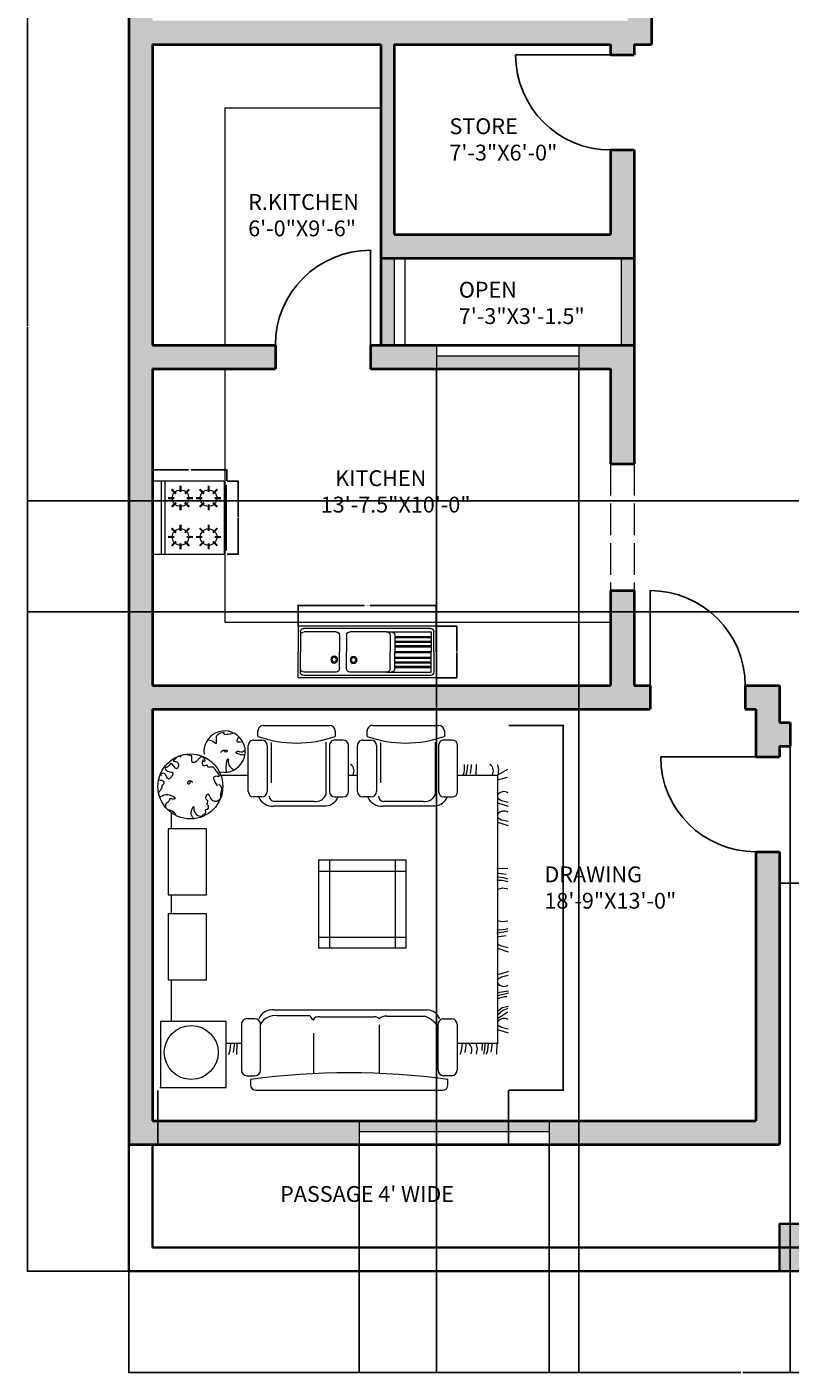
# Model space of a CAD drawing. Units: inches. Extents: x 2985 to 3527, y 3685 to 4528.
# Tile 1 of 5: x 2985 to 3274, y 3685 to 4195. Entities that reach past the tile are written whole.
import ezdxf

# ---------------------------------------------------------------- set-up
doc = ezdxf.new("R2010")
doc.units = ezdxf.units.IN
doc.linetypes.add('ACAD_ISO02W100', pattern=[15, 12, -3])
for name, color, linetype, lineweight in [('A-ANNO-DIMS', 2, 'Continuous', 18), ('A-AREA-IDEN', 7, 'Continuous', 25), ('A-EQPM', 8, 'Continuous', 18), ('A-FLOR-CASE', 9, 'Continuous', 20), ('A-FLOR-EDGE', 7, 'Continuous', 25), ('A-FLOR-FIXT', 9, 'Continuous', 18), ('A-FURN', 8, 'Continuous', 18), ('A-GLAZ', 4, 'Continuous', 18), ('A-SITE-WALL', 7, 'Continuous', 35), ('A-WALL', 7, 'Continuous', 40), ('A-WALL-OVHD', 7, 'ACAD_ISO02W100', 18), ('A-WALL-PATT', 8, 'Continuous', 13), ('door', 4, 'Continuous', 25)]:
    doc.layers.add(name, color=color, linetype=linetype, lineweight=lineweight)
doc.layers.add('A-GLAZ-PATT', color=241, linetype='Continuous', lineweight=13, true_color=0xf7abae)
doc.styles.get("Standard").update_dxf_attribs({"font": 'arial.ttf'})
doc.dimstyles.get("Standard").update_dxf_attribs({"dimtxt": 0.18, "dimasz": 0.18, "dimexe": 0.18, "dimexo": 0.0625, "dimgap": 0.09, "dimtad": 0, "dimtih": 1, "dimtoh": 1, "dimdec": 4, "dimzin": 0, "dimdsep": 46, "dimtxsty": 'Standard', "dimcen": 0.09, "dimadec": 0, "dimazin": 0, "dimtfac": 1, "dimtdec": 4, "dimtofl": 0, "dimtmove": 0, "dimatfit": 3, "dimfxl": 1, "dimtolj": 1, "dimtzin": 0, "dimarcsym": 0})

# ---------------------------------------------------------------- blocks, each defined once
blk = doc.blocks.new('A$C5E580471')
at = {"ltscale": 1000}
for p, q in [((0, 450), (0, 225)), ((1200, 450), (0, 450)), ((20, 400), (20, 225)), ((22, 370), (22, 225)), ((1150, 430), (50, 430)), ((331, 400), (52, 400)), ((361, 370), (361, 225)), ((421, 370), (421, 225)), ((770, 400), (451, 400)), ((770, 400), (1156, 400)), ((800, 370), (800, 225)), ((840, 370), (840, 225)), ((840, 360), (1156, 360)), ((1156, 400), (1156, 225)), ((1180, 225), (1180, 400)), ((1200, 225), (1200, 450)), ((840, 350), (1156, 350)), ((840, 320), (1156, 320)), ((840, 310), (1156, 310)), ((840, 280), (1156, 280)), ((840, 270), (1156, 270)), ((0, 0), (0, 225)), ((20, 50), (20, 225)), ((22, 80), (22, 225)), ((361, 80), (361, 225)), ((361, 80), (361, 225)), ((421, 80), (421, 225)), ((800, 80), (800, 225)), ((840, 230), (1156, 230)), ((840, 80), (840, 225)), ((840, 220), (1156, 220)), ((840, 180), (1156, 180)), ((840, 170), (1156, 170)), ((840, 140), (1156, 140)), ((840, 130), (1156, 130)), ((1156, 50), (1156, 225)), ((1180, 225), (1180, 50)), ((1200, 225), (1200, 0)), ((1200, 0), (0, 0)), ((1150, 20), (50, 20)), ((331, 50), (52, 50)), ((331, 50), (290, 50)), ((770, 50), (451, 50)), ((770, 50), (1156, 50)), ((840, 100), (1156, 100)), ((840, 90), (1156, 90))]:
    blk.add_line(p, q, dxfattribs=at)
for centre, radius in [((314, 292), 30), ((314, 292), 20), ((482, 295), 30), ((482, 295), 20)]:
    blk.add_circle(centre, radius, dxfattribs=at)
for centre, start, end in [((50, 400), 90, 180), ((52, 370), 90, 180), ((331, 370), 0, 90), ((451, 370), 90, 180), ((770, 370), 0, 90), ((810, 370), 0, 90), ((1150, 400), 0, 90), ((50, 50), 180, 270), ((52, 80), 180, 270), ((331, 80), 270, 0), ((331, 80), 270, 0), ((451, 80), 180, 270), ((770, 80), 270, 0), ((810, 80), 270, 0), ((1150, 50), 270, 0)]:
    blk.add_arc(centre, 30, start, end, dxfattribs=at)
blk = doc.blocks.new('A$C5A4E2756')
for p, q in [((0, 545), (610, 545)), ((0, 515), (610, 515))]:
    blk.add_line(p, q)
blk.add_lwpolyline([(0, 620), (0, 30, 0.414214), (10, 20), (600, 20, 0.414214), (610, 30), (610, 620)], format="xyb", close=True)
for points, const_width in [([(69, 461), (106, 424)], 17.3), ([(143, 491), (143, 439)], 17.3), ([(216, 461), (179, 424)], 17.3), ([(394, 461), (431, 424)], 17.3), ([(467, 491), (467, 439)], 17.3), ([(541, 461), (504, 424)], 17.3), ([(39, 387), (91, 387)], 17.3), ([(69, 314), (106, 351)], 17.3), ([(143, 284), (143, 335)], 17.3), ([(216, 314), (179, 351)], 17.3), ([(246, 387), (194, 387)], 17.3), ([(364, 387), (416, 387)], 17.3), ([(394, 314), (431, 351)], 17.3), ([(467, 284), (467, 335)], 17.3), ([(541, 314), (504, 351)], 17.3), ([(571, 387), (519, 387)], 17.3), ([(69, 227), (106, 190)], 17.3), ([(143, 257), (143, 205)], 17.3), ([(216, 227), (179, 190)], 17.3), ([(394, 227), (431, 190)], 17.3), ([(467, 257), (467, 205)], 17.3), ([(541, 227), (504, 190)], 17.3), ([(39, 153), (91, 153)], 17.3), ([(69, 80), (106, 117)], 17.3), ([(216, 80), (179, 117)], 17.3), ([(246, 153), (194, 153)], 17.3), ([(364, 153), (416, 153)], 17.3), ([(394, 80), (431, 117)], 17.3), ([(541, 80), (504, 117)], 17.3), ([(571, 153), (519, 153)], 17.3), ([(580, 5), (30, 5)], 10), ([(143, 50), (143, 101)], 17.3), ([(467, 50), (467, 101)], 17.3)]:
    blk.add_lwpolyline(points, dxfattribs=dict(const_width=const_width))
for centre in [(143, 387), (467, 387), (143, 153), (467, 153)]:
    blk.add_circle(centre, 69.1)
blk = doc.blocks.new('A$C688935E4')
for p, q in [((2302, 3327), (602, 3327)), ((519, 3194), (592, 3194)), ((552, 3277), (552, 3227)), ((2384, 3194), (2311, 3194)), ((2352, 3227), (2352, 3277)), ((3173, 3300), (2573, 3300)), ((2573, 3300), (2573, 2700)), ((3173, 2700), (3173, 3300)), ((469, 2725), (469, 3144)), ((642, 3144), (642, 2725)), ((1175, 3172), (1175, 2731)), ((1775, 3172), (1775, 2805)), ((2261, 3144), (2261, 2725)), ((2434, 2725), (2434, 3144)), ((108, 2997), (104, 2897)), ((158, 2980), (148, 2916)), ((189, 2960), (182, 2897)), ((200, 2997), (189, 2960)), ((240, 2963), (237, 2899)), ((291, 2997), (283, 2947)), ((283, 2947), (295, 2901)), ((396, 2982), (387, 2917)), ((428, 2962), (420, 2899)), ((439, 2999), (428, 2962)), ((2475, 2999), (2472, 2899)), ((2507, 2982), (2497, 2917)), ((2538, 2962), (2531, 2899)), ((2549, 2999), (2538, 2962)), ((97, 2899), (469, 2899)), ((102, 454), (102, 2904)), ((148, 2916), (148, 2899)), ((387, 2917), (387, 2901)), ((2434, 2899), (2573, 2899)), ((2497, 2917), (2497, 2901)), ((0, 2807), (98, 2776)), ((2, 2769), (65, 2754)), ((65, 2754), (100, 2733)), ((5, 2613), (101, 2675)), ((7, 2581), (51, 2600)), ((51, 2600), (101, 2642)), ((57, 2576), (99, 2607)), ((592, 2675), (519, 2675)), ((2140, 2593), (739, 2593)), ((1110, 2651), (768, 2651)), ((1721, 2656), (1224, 2656)), ((2108, 2646), (1810, 2646)), ((2311, 2675), (2384, 2675)), ((2573, 2700), (3173, 2700)), ((3071, 2700), (3071, 2319)), ((1, 2564), (57, 2576)), ((1, 2442), (101, 2465)), ((1, 2424), (103, 2437)), ((0, 2242), (98, 2274)), ((2, 2281), (65, 2296)), ((65, 2296), (100, 2316)), ((3103, 2319), (2753, 2319)), ((2753, 2319), (2753, 1719)), ((3103, 1719), (3103, 2319)), ((0, 2067), (98, 2035)), ((2, 2028), (65, 2013)), ((65, 2013), (100, 1993)), ((1732, 2029), (932, 2029)), ((932, 2029), (932, 1229)), ((1032, 1229), (1032, 2029)), ((1632, 1229), (1632, 2029)), ((1732, 1229), (1732, 2029)), ((6, 1875), (43, 1886)), ((23, 1918), (87, 1927)), ((43, 1886), (106, 1894)), ((87, 1927), (104, 1927)), ((1732, 1929), (932, 1929)), ((6, 1785), (56, 1792)), ((56, 1792), (102, 1781)), ((2753, 1719), (3103, 1719)), ((3071, 1719), (3071, 1543)), ((6, 1492), (56, 1484)), ((56, 1484), (102, 1495)), ((3103, 1543), (2753, 1543)), ((2753, 1543), (2753, 943)), ((3103, 943), (3103, 1543)), ((6, 1401), (43, 1390)), ((23, 1358), (87, 1349)), ((43, 1390), (106, 1382)), ((6, 1308), (106, 1305)), ((87, 1349), (104, 1349)), ((1732, 1329), (932, 1329)), ((932, 1229), (1732, 1229)), ((1632, 1229), (1632, 1229)), ((1732, 1329), (1732, 1329)), ((0, 916), (98, 885)), ((2, 877), (65, 862)), ((65, 862), (100, 842)), ((2753, 943), (3103, 943)), ((3071, 943), (3071, 797)), ((0, 740), (98, 709)), ((2, 701), (65, 686)), ((65, 686), (100, 666)), ((587, 652), (514, 652)), ((1146, 734), (670, 734)), ((670, 152), (670, 634)), ((775, 694), (1141, 694)), ((1254, 652), (1327, 652)), ((1582, 652), (1509, 652)), ((2141, 734), (1665, 734)), ((1665, 152), (1665, 634)), ((1770, 694), (2136, 694)), ((2249, 652), (2322, 652)), ((11, 473), (104, 500)), ((464, 602), (464, 183)), ((637, 183), (637, 602)), ((1167, 155), (1167, 522)), ((1204, 183), (1204, 602)), ((1377, 602), (1377, 183)), ((1459, 602), (1459, 183)), ((1632, 183), (1632, 602)), ((2162, 155), (2162, 522)), ((2199, 183), (2199, 602)), ((2372, 602), (2372, 183)), ((9, 402), (102, 454)), ((95, 455), (88, 405)), ((88, 405), (99, 359)), ((464, 454), (102, 454)), ((296, 455), (292, 355)), ((346, 438), (336, 374)), ((336, 374), (336, 357)), ((377, 418), (370, 355)), ((388, 455), (377, 418)), ((1459, 454), (1377, 454)), ((2621, 454), (2372, 454)), ((514, 133), (587, 133)), ((1327, 133), (1254, 133)), ((1509, 133), (1582, 133)), ((2322, 133), (2249, 133)), ((585, 50), (585, 100)), ((1239, 0), (635, 0)), ((1289, 100), (1289, 50)), ((1580, 50), (1580, 100)), ((2234, 0), (1630, 0)), ((2284, 100), (2284, 50))]:
    blk.add_line(p, q)
for centre, radius in [((2892, 2982), 246), ((2900, 556), 296)]:
    blk.add_circle(centre, radius)
for centre, radius, start, end in [((602, 3277), 50, 90, 180), ((2302, 3277), 50, 0, 90), ((519, 3144), 50, 90, 180), ((1452, 9941), 6774, 262.3653, 277.6347), ((592, 3144), 50, 0, 90), ((2311, 3144), 50, 90, 180), ((2384, 3144), 50, 0, 90), ((469, 2919), 256, 162.3499, 184.9697), ((408, 2957), 73.8, 148.9813, 234.4689), ((40, 2745), 73.8, 238.9813, 324.4689), ((519, 2725), 50, 180, 270), ((592, 2725), 50, 270, 0), ((860, 2910), 275, 218.1017, 250.3904), ((2129, 2794), 149, 261.7696, 332.5418), ((2311, 2725), 50, 180, 270), ((2384, 2725), 50, 270, 0), ((747, 2722), 129, 201.1539, 266.4257), ((1120, 2733), 82.5, 263.0888, 316.219), ((1220, 2706), 50.3, 216.9828, 275.0921), ((1731, 2711), 55.5, 259.6951, 333.4351), ((1716, 2606), 102, 22.8336, 50.9061), ((2153, 2725), 133, 264.3783, 337.7856), ((21, 2635), 161, 268.1865, 300.459), ((40, 2305), 73.8, 35.5311, 121.0187), ((84, 1607), 256, 85.0303, 107.6501), ((84, 1669), 256, 252.3499, 274.9697), ((40, 854), 73.8, 238.9813, 324.4689), ((40, 677), 73.8, 238.9813, 324.4689), ((514, 602), 50, 90, 180), ((679, 605), 129, 93.5743, 158.8461), ((587, 602), 50, 0, 90), ((765, 589), 105, 84.6221, 154.8677), ((1134, 643), 51.7, 0.1551, 82.6921), ((1159, 602), 133, 22.2144, 95.6217), ((1254, 602), 50, 90, 180), ((1327, 602), 50, 0, 90), ((1509, 602), 50, 90, 180), ((1674, 605), 129, 93.5743, 158.8461), ((1582, 602), 50, 0, 90), ((1760, 589), 105, 84.6221, 154.8677), ((2129, 643), 51.7, 0.1551, 82.6921), ((2154, 602), 133, 22.2144, 95.6217), ((2249, 602), 50, 90, 180), ((2322, 602), 50, 0, 90), ((212, 415), 73.8, 148.9813, 234.4689), ((656, 377), 256, 162.3499, 184.9697), ((1482, 415), 73.8, 148.9813, 234.4689), ((2588, 238), 188, 79.0531, 7.4753), ((514, 183), 50, 180, 270), ((937, -899), 1059, 70.6126, 109.3874), ((587, 183), 50, 270, 0), ((1254, 183), 50, 180, 270), ((1327, 183), 50, 270, 0), ((1509, 183), 50, 180, 270), ((1932, -899), 1059, 70.6126, 109.3874), ((1582, 183), 50, 270, 0), ((2249, 183), 50, 180, 270), ((2322, 183), 50, 270, 0), ((635, 50), 50, 180, 270), ((1239, 50), 50, 270, 0), ((1630, 50), 50, 180, 270), ((2234, 50), 50, 270, 0)]:
    blk.add_arc(centre, radius, start, end)
for points, knots in [([(2872, 845), (2883, 832), (2907, 803), (2861, 711), (2881, 801), (2803, 845), (2776, 806), (2751, 796), (2769, 759), (2736, 767), (2735, 745), (2735, 729), (2757, 717), (2729, 687), (2772, 671), (2738, 597), (2722, 670), (2689, 689), (2654, 692), (2636, 677), (2616, 660), (2630, 618), (2602, 571), (2628, 547), (2640, 536)], [0, 0, 0, 0, 51.917432, 115.953134, 148.653762, 243.503618, 260.320221, 285.545105, 312.300159, 330.382893, 349.184414, 364.34271, 376.955185, 410.191929, 431.212679, 481.045637, 526.423186, 566.857378, 599.557953, 620.994965, 633.607388, 678.298148, 729.616372, 774.208118, 774.208118, 774.208118, 774.208118]), ([(3193, 497), (3171, 498), (3139, 498), (3141, 537), (3162, 543), (3158, 564), (3172, 582), (3178, 600), (3200, 616), (3176, 666), (3127, 605), (3003, 663), (3064, 677), (3088, 658), (3091, 699), (3124, 704), (3131, 738), (3113, 769), (3068, 773), (3045, 796), (3032, 809)], [0, 0, 0, 0, 53.592527, 74.613275, 89.477172, 107.559926, 127.501946, 155.547132, 163.955427, 205.361526, 244.007616, 348.394114, 372.361442, 391.162931, 417.7523, 451.647222, 476.161445, 506.768106, 548.174139, 601.102996, 601.102996, 601.102996, 601.102996]), ([(2931, 265), (2913, 268), (2875, 273), (2902, 335), (2834, 339), (2809, 262), (2771, 299), (2764, 331), (2787, 328), (2779, 303), (2799, 340), (2788, 367), (2763, 368), (2743, 356), (2748, 379), (2722, 378), (2690, 370), (2672, 410), (2651, 432), (2622, 472), (2715, 450), (2679, 509), (2655, 551)], [0, 0, 0, 0, 45.280034, 92.937377, 119.85705, 202.50888, 236.142072, 256.951553, 269.208667, 281.099788, 301.041808, 334.936757, 361.691781, 371.092526, 386.250821, 398.507936, 434.181286, 480.617605, 503.835785, 537.072526, 575.832818, 664.519513, 664.519513, 664.519513, 664.519513]), ([(2881, 521), (2889, 512), (2904, 496), (2937, 526), (2907, 537), (2904, 518), (2889, 500), (2884, 512), (2881, 518)], [0, 0, 0, 0, 30.606664, 58.014358, 74.023252, 91.35741, 108.174033, 123.037946, 123.037946, 123.037946, 123.037946]), ([(2569, 423), (2572, 410), (2581, 375), (2552, 269), (2560, 365), (2529, 386), (2509, 399)], [0, 0, 0, 0, 44.986397, 121.416439, 163.141462, 232.795961, 232.795961, 232.795961, 232.795961]), ([(2985, 289), (2992, 285), (3013, 272), (3030, 301), (3066, 331), (2996, 318), (3019, 448), (3076, 310), (3098, 385), (3133, 380), (3121, 432), (3022, 404), (3112, 529), (3118, 434), (3165, 434), (3170, 452), (3172, 461)], [0, 0, 0, 0, 22.639985, 64.891145, 88.109294, 118.425777, 183.827032, 255.421062, 303.81444, 318.972681, 339.993429, 410.655563, 480.815761, 542.675345, 566.457594, 593.046986, 593.046986, 593.046986, 593.046986]), ([(2402, 271), (2418, 270), (2442, 269), (2493, 249), (2462, 227), (2432, 251), (2412, 232), (2402, 224)], [0, 0, 0, 0, 54.24811, 86.403653, 101.26755, 140.368354, 175.036649, 175.036649, 175.036649, 175.036649]), ([(2622, 247), (2617, 239), (2606, 219), (2549, 226), (2578, 251), (2587, 229), (2599, 231), (2604, 232)], [0, 0, 0, 0, 29.429031, 69.090853, 83.95475, 102.989865, 117.853741, 117.853741, 117.853741, 117.853741]), ([(2465, 111), (2472, 124), (2489, 155), (2451, 149), (2429, 146)], [0, 0, 0, 0, 34.795552, 82.452812, 82.452812, 82.452812, 82.452812]), ([(2738, 131), (2718, 133), (2692, 135), (2662, 180), (2660, 126), (2665, 84), (2627, 67), (2592, 61), (2601, 83), (2552, 80), (2529, 73), (2512, 69)], [0, 0, 0, 0, 60.194174, 81.21491, 114.451654, 156.176677, 217.38995, 226.308276, 238.199396, 262.71358, 323.346586, 323.346586, 323.346586, 323.346586])]:
    blk.add_open_spline(points, degree=3, knots=knots)
blk.add_point((3173, 3300))
blk = doc.blocks.new('DOOR-SWING-36IN')
blk.add_line((0, 0), (0, 36))
blk.add_arc((0, 0), 36, 0, 90)
blk = doc.blocks.new('GATE-PIER-18IN')
h = blk.add_hatch(color=256)
h.dxf.hatch_style = 1
h.paths.add_polyline_path([(18, 0), (18, 18), (0, 18), (0, 0)])
blk.add_lwpolyline([(0, 0), (18, 0), (18, 18), (0, 18)], close=True)
blk = doc.blocks.new('*D32')
at = {"layer": 'A-ANNO-DIMS', "color": 0, "lineweight": -2, "transparency": 16777216}
for p, q in [((3087.95, 3967.98), (3087.95, 3975.94)), ((3088.13, 3975.76), (3112.97, 3975.76)), ((3140.07, 3975.76), (3115.23, 3975.76)), ((3140.25, 3967.98), (3140.25, 3975.94))]:
    blk.add_line(p, q, dxfattribs=at)
at = {"layer": 'A-ANNO-DIMS', "color": 0, "transparency": 16777216}
for points in [[(3088.13, 3975.79), (3088.13, 3975.73), (3087.95, 3975.76)], [(3140.07, 3975.79), (3140.07, 3975.73), (3140.25, 3975.76)]]:
    blk.add_solid(points, dxfattribs=at)
at = {"layer": 'Defpoints', "color": 0, "transparency": 16777216}
for p in [(3140.25, 3975.76), (3087.95, 3967.92), (3140.25, 3967.92)]:
    blk.add_point(p, dxfattribs=at)
at = {"layer": 'A-ANNO-DIMS', "color": 0, "transparency": 16777216, "insert": (3114.1, 3975.76), "char_height": 0.18, "attachment_point": 5}
blk.add_mtext('\\A1;KITCHEN SINK 52', dxfattribs=at)
blk = doc.blocks.new('*D33')
at = {"layer": 'A-ANNO-DIMS', "color": 0, "lineweight": -2, "transparency": 16777216}
for p, q in [((3140.31, 3967.92), (3148.28, 3967.92)), ((3148.1, 3967.74), (3148.1, 3958.29)), ((3148.1, 3948.49), (3148.1, 3957.93)), ((3140.31, 3948.31), (3148.28, 3948.31))]:
    blk.add_line(p, q, dxfattribs=at)
at = {"layer": 'A-ANNO-DIMS', "color": 0, "transparency": 16777216}
for points in [[(3148.07, 3967.74), (3148.13, 3967.74), (3148.1, 3967.92)], [(3148.07, 3948.49), (3148.13, 3948.49), (3148.1, 3948.31)]]:
    blk.add_solid(points, dxfattribs=at)
at = {"layer": 'Defpoints', "color": 0, "transparency": 16777216}
for p in [(3140.25, 3967.92), (3140.25, 3948.31), (3148.1, 3948.31)]:
    blk.add_point(p, dxfattribs=at)
at = {"layer": 'A-ANNO-DIMS', "color": 0, "transparency": 16777216, "insert": (3148.1, 3958.11), "char_height": 0.18, "attachment_point": 5}
blk.add_mtext('\\A1;20', dxfattribs=at)
blk = doc.blocks.new('*D34')
at = {"layer": 'A-ANNO-DIMS', "color": 0, "lineweight": -2, "transparency": 16777216}
for p, q in [((3032.83, 4022.95), (3032.83, 4027.29)), ((3033.01, 4027.11), (3046.39, 4027.11)), ((3060.8, 4027.11), (3047.43, 4027.11)), ((3060.98, 4022.95), (3060.98, 4027.29))]:
    blk.add_line(p, q, dxfattribs=at)
at = {"layer": 'A-ANNO-DIMS', "color": 0, "transparency": 16777216}
for points in [[(3033.01, 4027.14), (3033.01, 4027.08), (3032.83, 4027.11)], [(3060.8, 4027.14), (3060.8, 4027.08), (3060.98, 4027.11)]]:
    blk.add_solid(points, dxfattribs=at)
at = {"layer": 'Defpoints', "color": 0, "transparency": 16777216}
for p in [(3032.83, 4027.11), (3032.83, 4022.89), (3060.98, 4022.89)]:
    blk.add_point(p, dxfattribs=at)
at = {"layer": 'A-ANNO-DIMS', "color": 0, "transparency": 16777216, "insert": (3046.91, 4027.11), "char_height": 0.18, "attachment_point": 5}
blk.add_mtext('\\A1;HOB 28', dxfattribs=at)
blk = doc.blocks.new('*D35')
at = {"layer": 'A-ANNO-DIMS', "color": 0, "lineweight": -2, "transparency": 16777216}
for p, q in [((3061.04, 4022.89), (3065.38, 4022.89)), ((3065.2, 4022.71), (3065.2, 4009.23)), ((3065.2, 3995.38), (3065.2, 4008.86)), ((3061.04, 3995.2), (3065.38, 3995.2))]:
    blk.add_line(p, q, dxfattribs=at)
at = {"layer": 'A-ANNO-DIMS', "color": 0, "transparency": 16777216}
for points in [[(3065.17, 4022.71), (3065.23, 4022.71), (3065.2, 4022.89)], [(3065.17, 3995.38), (3065.23, 3995.38), (3065.2, 3995.2)]]:
    blk.add_solid(points, dxfattribs=at)
at = {"layer": 'Defpoints', "color": 0, "transparency": 16777216}
for p in [(3060.98, 4022.89), (3065.2, 4022.89), (3060.98, 3995.2)]:
    blk.add_point(p, dxfattribs=at)
at = {"layer": 'A-ANNO-DIMS', "color": 0, "transparency": 16777216, "insert": (3065.2, 4009.05), "char_height": 0.18, "attachment_point": 5}
blk.add_mtext('\\A1;28', dxfattribs=at)
blk = doc.blocks.new('*D36')
at = {"layer": 'A-ANNO-DIMS', "color": 0, "lineweight": -2, "transparency": 16777216}
for p, q in [((3167.74, 3930.25), (3188.6, 3930.25)), ((3188.42, 3930.07), (3188.42, 3861.29)), ((3188.42, 3792.14), (3188.42, 3860.92)), ((3167.74, 3791.96), (3188.6, 3791.96))]:
    blk.add_line(p, q, dxfattribs=at)
at = {"layer": 'A-ANNO-DIMS', "color": 0, "transparency": 16777216}
for points in [[(3188.39, 3930.07), (3188.45, 3930.07), (3188.42, 3930.25)], [(3188.39, 3792.14), (3188.45, 3792.14), (3188.42, 3791.96)]]:
    blk.add_solid(points, dxfattribs=at)
at = {"layer": 'Defpoints', "color": 0, "transparency": 16777216}
for p in [(3167.68, 3930.25), (3167.68, 3791.96), (3188.42, 3791.96)]:
    blk.add_point(p, dxfattribs=at)
at = {"layer": 'A-ANNO-DIMS', "color": 0, "transparency": 16777216, "insert": (3188.42, 3861.1), "char_height": 0.18, "attachment_point": 5}
blk.add_mtext('\\A1;SEATING GROUP 138', dxfattribs=at)
blk = doc.blocks.new('*D37')
at = {"layer": 'A-ANNO-DIMS', "color": 0, "lineweight": -2, "transparency": 16777216}
for p, q in [((3034.76, 3791.9), (3034.76, 3771.04)), ((3167.68, 3791.9), (3167.68, 3771.04)), ((3034.94, 3771.22), (3100.94, 3771.22)), ((3167.5, 3771.22), (3101.5, 3771.22))]:
    blk.add_line(p, q, dxfattribs=at)
at = {"layer": 'A-ANNO-DIMS', "color": 0, "transparency": 16777216}
for points in [[(3034.94, 3771.25), (3034.94, 3771.19), (3034.76, 3771.22)], [(3167.5, 3771.25), (3167.5, 3771.19), (3167.68, 3771.22)]]:
    blk.add_solid(points, dxfattribs=at)
at = {"layer": 'Defpoints', "color": 0, "transparency": 16777216}
for p in [(3034.76, 3791.96), (3167.68, 3791.96), (3034.76, 3771.22)]:
    blk.add_point(p, dxfattribs=at)
at = {"layer": 'A-ANNO-DIMS', "color": 0, "transparency": 16777216, "insert": (3101.22, 3771.22), "char_height": 0.18, "attachment_point": 5}
blk.add_mtext('\\A1;133', dxfattribs=at)
blk = doc.blocks.new('*D40')
at = {"layer": 'A-ANNO-DIMS', "color": 0, "lineweight": -2, "transparency": 16777216}
for p, q in [((3023.83, 3723.31), (3023.83, 3684.79)), ((3488.33, 3723.31), (3488.33, 3684.79)), ((3024.01, 3684.97), (3255.69, 3684.97)), ((3488.15, 3684.97), (3256.48, 3684.97))]:
    blk.add_line(p, q, dxfattribs=at)
at = {"layer": 'A-ANNO-DIMS', "color": 0, "transparency": 16777216}
for points in [[(3024.01, 3685), (3024.01, 3684.94), (3023.83, 3684.97)], [(3488.15, 3685), (3488.15, 3684.94), (3488.33, 3684.97)]]:
    blk.add_solid(points, dxfattribs=at)
at = {"layer": 'Defpoints', "color": 0, "transparency": 16777216}
for p in [(3023.83, 3723.37), (3488.33, 3723.37), (3488.33, 3684.97)]:
    blk.add_point(p, dxfattribs=at)
at = {"layer": 'A-ANNO-DIMS', "color": 0, "transparency": 16777216, "insert": (3256.08, 3684.97), "char_height": 0.18, "attachment_point": 5}
blk.add_mtext('\\A1;464.5', dxfattribs=at)
blk = doc.blocks.new('*D41')
at = {"layer": 'A-ANNO-DIMS', "color": 0, "lineweight": -2, "transparency": 16777216}
for p, q in [((3023.77, 4439.37), (2985.25, 4439.37)), ((2985.43, 4439.19), (2985.43, 4081.55)), ((2985.43, 3723.55), (2985.43, 4081.19)), ((3023.77, 3723.37), (2985.25, 3723.37))]:
    blk.add_line(p, q, dxfattribs=at)
at = {"layer": 'A-ANNO-DIMS', "color": 0, "transparency": 16777216}
for points in [[(2985.4, 4439.19), (2985.46, 4439.19), (2985.43, 4439.37)], [(2985.4, 3723.55), (2985.46, 3723.55), (2985.43, 3723.37)]]:
    blk.add_solid(points, dxfattribs=at)
at = {"layer": 'Defpoints', "color": 0, "transparency": 16777216}
for p in [(2985.43, 4439.37), (3023.83, 4439.37), (3023.83, 3723.37)]:
    blk.add_point(p, dxfattribs=at)
at = {"layer": 'A-ANNO-DIMS', "color": 0, "transparency": 16777216, "insert": (2985.43, 4081.37), "char_height": 0.18, "attachment_point": 5}
blk.add_mtext('\\A1;716', dxfattribs=at)
blk = doc.blocks.new('*D51')
at = {"layer": 'A-ANNO-DIMS', "color": 0, "lineweight": -2, "transparency": 16777216}
for p, q in [((3274.33, 3931.31), (3274.33, 3684.79)), ((3346.33, 3931.31), (3346.33, 3684.79)), ((3274.51, 3684.97), (3310.12, 3684.97)), ((3346.15, 3684.97), (3310.55, 3684.97))]:
    blk.add_line(p, q, dxfattribs=at)
at = {"layer": 'A-ANNO-DIMS', "color": 0, "transparency": 16777216}
for points in [[(3274.51, 3685), (3274.51, 3684.94), (3274.33, 3684.97)], [(3346.15, 3685), (3346.15, 3684.94), (3346.33, 3684.97)]]:
    blk.add_solid(points, dxfattribs=at)
at = {"layer": 'Defpoints', "color": 0, "transparency": 16777216}
for p in [(3274.33, 3931.37), (3346.33, 3931.37), (3346.33, 3684.97)]:
    blk.add_point(p, dxfattribs=at)
at = {"layer": 'A-ANNO-DIMS', "color": 0, "transparency": 16777216, "insert": (3310.33, 3684.97), "char_height": 0.18, "attachment_point": 5}
blk.add_mtext('\\A1;72', dxfattribs=at)
blk = doc.blocks.new('*D52')
at = {"layer": 'A-ANNO-DIMS', "color": 0, "lineweight": -2, "transparency": 16777216}
for p, q in [((3342.27, 4015.37), (2985.25, 4015.37)), ((2985.43, 4015.19), (2985.43, 3994.55)), ((2985.43, 3973.55), (2985.43, 3994.19)), ((3342.27, 3973.37), (2985.25, 3973.37))]:
    blk.add_line(p, q, dxfattribs=at)
at = {"layer": 'A-ANNO-DIMS', "color": 0, "transparency": 16777216}
for points in [[(2985.4, 4015.19), (2985.46, 4015.19), (2985.43, 4015.37)], [(2985.4, 3973.55), (2985.46, 3973.55), (2985.43, 3973.37)]]:
    blk.add_solid(points, dxfattribs=at)
at = {"layer": 'Defpoints', "color": 0, "transparency": 16777216}
for p in [(2985.43, 4015.37), (3342.33, 4015.37), (3342.33, 3973.37)]:
    blk.add_point(p, dxfattribs=at)
at = {"layer": 'A-ANNO-DIMS', "color": 0, "transparency": 16777216, "insert": (2985.43, 3994.37), "char_height": 0.18, "attachment_point": 5}
blk.add_mtext('\\A1;42', dxfattribs=at)
blk = doc.blocks.new('*D57')
at = {"layer": 'A-ANNO-DIMS', "color": 0, "lineweight": -2, "transparency": 16777216}
for p, q in [((3111.08, 3771.31), (3111.08, 3684.79)), ((3183.08, 3771.31), (3183.08, 3684.79)), ((3111.26, 3684.97), (3146.87, 3684.97)), ((3182.9, 3684.97), (3147.3, 3684.97))]:
    blk.add_line(p, q, dxfattribs=at)
at = {"layer": 'A-ANNO-DIMS', "color": 0, "transparency": 16777216}
for points in [[(3111.26, 3685), (3111.26, 3684.94), (3111.08, 3684.97)], [(3182.9, 3685), (3182.9, 3684.94), (3183.08, 3684.97)]]:
    blk.add_solid(points, dxfattribs=at)
at = {"layer": 'Defpoints', "color": 0, "transparency": 16777216}
for p in [(3111.08, 3771.37), (3183.08, 3771.37), (3183.08, 3684.97)]:
    blk.add_point(p, dxfattribs=at)
at = {"layer": 'A-ANNO-DIMS', "color": 0, "transparency": 16777216, "insert": (3147.08, 3684.97), "char_height": 0.18, "attachment_point": 5}
blk.add_mtext('\\A1;72', dxfattribs=at)
blk = doc.blocks.new('*D58')
at = {"layer": 'A-ANNO-DIMS', "color": 0, "lineweight": -2, "transparency": 16777216}
for p, q in [((3023.83, 3771.31), (3023.83, 3684.79)), ((3111.08, 3771.31), (3111.08, 3684.79)), ((3024.01, 3684.97), (3067.06, 3684.97)), ((3110.9, 3684.97), (3067.85, 3684.97))]:
    blk.add_line(p, q, dxfattribs=at)
at = {"layer": 'A-ANNO-DIMS', "color": 0, "transparency": 16777216}
for points in [[(3024.01, 3685), (3024.01, 3684.94), (3023.83, 3684.97)], [(3110.9, 3685), (3110.9, 3684.94), (3111.08, 3684.97)]]:
    blk.add_solid(points, dxfattribs=at)
at = {"layer": 'Defpoints', "color": 0, "transparency": 16777216}
for p in [(3023.83, 3771.37), (3111.08, 3771.37), (3111.08, 3684.97)]:
    blk.add_point(p, dxfattribs=at)
at = {"layer": 'A-ANNO-DIMS', "color": 0, "transparency": 16777216, "insert": (3067.46, 3684.97), "char_height": 0.18, "attachment_point": 5}
blk.add_mtext('\\A1;87.25', dxfattribs=at)
blk = doc.blocks.new('*D59')
at = {"layer": 'A-ANNO-DIMS', "color": 0, "lineweight": -2, "transparency": 16777216}
for p, q in [((3140.33, 4065.31), (3140.33, 3684.79)), ((3194.33, 4065.31), (3194.33, 3684.79)), ((3140.51, 3684.97), (3167.11, 3684.97)), ((3194.15, 3684.97), (3167.55, 3684.97))]:
    blk.add_line(p, q, dxfattribs=at)
at = {"layer": 'A-ANNO-DIMS', "color": 0, "transparency": 16777216}
for points in [[(3140.51, 3685), (3140.51, 3684.94), (3140.33, 3684.97)], [(3194.15, 3685), (3194.15, 3684.94), (3194.33, 3684.97)]]:
    blk.add_solid(points, dxfattribs=at)
at = {"layer": 'Defpoints', "color": 0, "transparency": 16777216}
for p in [(3140.33, 4065.37), (3194.33, 4065.37), (3194.33, 3684.97)]:
    blk.add_point(p, dxfattribs=at)
at = {"layer": 'A-ANNO-DIMS', "color": 0, "transparency": 16777216, "insert": (3167.33, 3684.97), "char_height": 0.18, "attachment_point": 5}
blk.add_mtext('\\A1;54', dxfattribs=at)

msp = doc.modelspace()

# ---------------------------------------------------------------- hatches: boundary and pattern name
at = {"layer": 'A-GLAZ-PATT'}
h = msp.add_hatch(color=256, dxfattribs=at)
h.dxf.hatch_style = 1
h.paths.add_polyline_path([(3124.333, 4107.372), (3119.333, 4107.372), (3119.333, 4074.372), (3124.333, 4074.372)])
h = msp.add_hatch(color=256, dxfattribs=at)
h.dxf.hatch_style = 1
h.paths.add_polyline_path([(3215.333, 4107.372), (3210.333, 4107.372), (3210.333, 4074.372), (3215.333, 4074.372)])
h = msp.add_hatch(color=256, dxfattribs=at)
h.dxf.hatch_style = 1
h.paths.add_polyline_path([(3194.333, 4070.372), (3140.333, 4070.372), (3140.333, 4065.372), (3194.333, 4065.372)])
h = msp.add_hatch(color=256, dxfattribs=at)
h.dxf.hatch_style = 1
h.paths.add_polyline_path([(3183.083, 3780.372), (3111.083, 3780.372), (3111.083, 3776.372), (3183.083, 3776.372)])
at = {"layer": 'A-WALL-PATT'}
h = msp.add_hatch(color=256, dxfattribs=at)
h.dxf.hatch_style = 1
h.paths.add_polyline_path([(3023.833, 4065.372), (3023.833, 3771.372), (3111.083, 3771.372), (3111.083, 3780.372), (3032.833, 3780.372), (3032.833, 3936.372), (3221.333, 3936.372), (3221.333, 3945.372), (3215.333, 3945.372), (3215.333, 3981.372), (3206.333, 3981.372), (3206.333, 3945.372), (3032.833, 3945.372), (3032.833, 4065.372), (3079.333, 4065.372), (3079.333, 4074.372), (3032.833, 4074.372), (3032.833, 4188.372), (3119.333, 4188.372), (3119.333, 4107.372), (3215.333, 4107.372), (3215.333, 4148.372), (3206.333, 4148.372), (3206.333, 4116.372), (3124.333, 4116.372), (3124.333, 4188.372), (3206.333, 4188.372), (3206.333, 4184.372), (3215.333, 4184.372), (3215.333, 4188.372), (3221.833, 4188.372), (3221.833, 4201.372), (3212.833, 4201.372), (3212.833, 4197.372), (3032.833, 4197.372), (3032.833, 4353.372), (3068.479, 4353.372), (3068.479, 4358.372), (3032.833, 4358.372), (3032.833, 4430.372), (3137.833, 4430.372), (3137.833, 4404.372), (3137.833, 4392.372), (3142.833, 4392.372), (3142.833, 4430.372), (3190.833, 4430.372), (3190.833, 4439.372), (3023.833, 4439.372)])
h = msp.add_hatch(color=256, dxfattribs=at)
h.dxf.hatch_style = 1
h.paths.add_polyline_path([(3140.333, 4074.372), (3115.333, 4074.372), (3115.333, 4065.372), (3140.333, 4065.372)])
h = msp.add_hatch(color=256, dxfattribs=at)
h.dxf.hatch_style = 1
h.paths.add_polyline_path([(3215.333, 4074.372), (3194.333, 4074.372), (3194.333, 4065.372), (3206.333, 4065.372), (3206.333, 4029.372), (3215.333, 4029.372)])
h = msp.add_hatch(color=256, dxfattribs=at)
h.dxf.hatch_style = 1
h.paths.add_polyline_path([(3274.333, 3931.372), (3270.333, 3931.372), (3270.333, 3945.372), (3257.333, 3945.372), (3257.333, 3936.372), (3261.333, 3936.372), (3261.333, 3918.372), (3270.333, 3918.372), (3270.333, 3922.372), (3274.333, 3922.372)])
h = msp.add_hatch(color=256, dxfattribs=at)
h.dxf.hatch_style = 1
h.paths.add_polyline_path([(3270.333, 3882.372), (3261.333, 3882.372), (3261.333, 3780.372), (3183.083, 3780.372), (3183.083, 3771.372), (3270.333, 3771.372)])

# ---------------------------------------------------------------- linework, layer by layer
at = {"layer": 'A-FLOR-CASE'}
for p, q in [((3060.174, 4164.372), (3119.333, 4164.372)), ((3060.174, 4164.372), (3060.174, 4074.372)), ((3060.174, 4065.372), (3060.174, 3969.372)), ((3060.174, 3969.372), (3206.333, 3969.372))]:
    msp.add_line(p, q, dxfattribs=at)
at = {"layer": 'A-FLOR-EDGE'}
msp.add_line((3270.333, 3870.449), (3282.333, 3870.449), dxfattribs=at)
at = {"layer": 'A-GLAZ'}
for p, q in [((3124.333, 4107.372), (3124.333, 4074.372)), ((3128.333, 4107.372), (3128.333, 4074.372)), ((3210.333, 4107.372), (3210.333, 4074.372)), ((3140.333, 4074.372), (3140.333, 4065.372)), ((3194.333, 4074.372), (3194.333, 4065.372)), ((3140.333, 4070.372), (3194.333, 4070.372)), ((3111.083, 3780.372), (3111.083, 3771.372)), ((3111.083, 3776.372), (3183.083, 3776.372)), ((3183.083, 3780.372), (3183.083, 3771.372))]:
    msp.add_line(p, q, dxfattribs=at)
at = {"layer": 'A-SITE-WALL'}
for p, q in [((3023.833, 3771.372), (3023.833, 3723.372)), ((3032.833, 3771.372), (3032.833, 3732.372)), ((3270.333, 3741.372), (3270.333, 3723.372)), ((3032.833, 3732.372), (3288.333, 3732.372)), ((3023.833, 3723.372), (3288.333, 3723.372))]:
    msp.add_line(p, q, dxfattribs=at)
at = {"layer": 'A-WALL'}
for p, q in [((3023.833, 4439.372), (3023.833, 4065.372)), ((3221.833, 4201.372), (3221.833, 4188.372)), ((3032.833, 4188.372), (3119.333, 4188.372)), ((3032.833, 4188.372), (3032.833, 4074.372)), ((3119.333, 4188.372), (3119.333, 4074.372)), ((3124.333, 4188.372), (3124.333, 4116.372)), ((3124.333, 4188.372), (3206.333, 4188.372)), ((3206.333, 4188.372), (3206.333, 4184.372)), ((3206.333, 4184.372), (3215.333, 4184.372)), ((3215.333, 4188.372), (3215.333, 4184.372)), ((3215.333, 4188.372), (3221.833, 4188.372)), ((3206.333, 4148.372), (3215.333, 4148.372)), ((3206.333, 4148.372), (3206.333, 4116.372)), ((3215.333, 4148.372), (3215.333, 4029.372)), ((3124.333, 4116.372), (3206.333, 4116.372)), ((3119.333, 4107.372), (3215.333, 4107.372)), ((3032.833, 4074.372), (3079.333, 4074.372)), ((3079.333, 4074.372), (3079.333, 4065.372)), ((3115.333, 4074.372), (3115.333, 4065.372)), ((3115.333, 4074.372), (3215.333, 4074.372)), ((3023.833, 4065.372), (3023.833, 3771.372)), ((3032.833, 4065.372), (3079.333, 4065.372)), ((3032.833, 4065.372), (3032.833, 3945.372)), ((3115.333, 4065.372), (3206.333, 4065.372)), ((3206.333, 4065.372), (3206.333, 4029.372)), ((3206.333, 4029.372), (3215.333, 4029.372)), ((3206.333, 3981.372), (3215.333, 3981.372)), ((3206.333, 3981.372), (3206.333, 3945.372)), ((3215.333, 3981.372), (3215.333, 3945.372)), ((3032.833, 3945.372), (3206.333, 3945.372)), ((3215.333, 3945.372), (3221.333, 3945.372)), ((3221.333, 3945.372), (3221.333, 3936.372)), ((3257.333, 3945.372), (3257.333, 3936.372)), ((3257.333, 3945.372), (3270.333, 3945.372)), ((3270.333, 3945.372), (3270.333, 3931.372)), ((3032.833, 3936.372), (3221.333, 3936.372)), ((3032.833, 3936.372), (3032.833, 3780.372)), ((3257.333, 3936.372), (3261.333, 3936.372)), ((3261.333, 3936.372), (3261.333, 3918.372)), ((3270.333, 3931.372), (3274.333, 3931.372)), ((3274.333, 3931.372), (3274.333, 3922.372)), ((3270.333, 3922.372), (3274.333, 3922.372)), ((3270.333, 3922.372), (3270.333, 3918.372)), ((3261.333, 3918.372), (3270.333, 3918.372)), ((3261.333, 3882.372), (3270.333, 3882.372)), ((3261.333, 3882.372), (3261.333, 3780.372)), ((3270.333, 3882.372), (3270.333, 3771.372)), ((3032.833, 3780.372), (3261.333, 3780.372)), ((3023.833, 3771.372), (3270.333, 3771.372))]:
    msp.add_line(p, q, dxfattribs=at)
at = {"layer": 'A-WALL-OVHD'}
for p, q in [((3206.333, 4029.372), (3206.333, 3981.372)), ((3215.333, 4029.372), (3215.333, 3981.372))]:
    msp.add_line(p, q, dxfattribs=at)

# ---------------------------------------------------------------- block references
at = {"layer": 'A-EQPM', "xscale": 0.0453978231806992, "yscale": 0.0453978231806992, "zscale": 0.0453978231806992, "rotation": 90}
msp.add_blockref('A$C5A4E2756', (3060.98, 3995.199), dxfattribs=at)
at = {"layer": 'A-FLOR-FIXT', "xscale": -0.0435718197915921, "yscale": 0.0435718197915921, "zscale": 0.0435718197915921, "rotation": 180}
msp.add_blockref('A$C5E580471', (3087.95, 3967.916), dxfattribs=at)
at = {"layer": 'A-FURN', "xscale": 0.0415652994726084, "yscale": 0.0415652994726084, "zscale": 0.0415652994726084, "rotation": 180}
msp.add_blockref('A$C688935E4', (3167.677, 3930.245), dxfattribs=at)
at = {"layer": 'A-SITE-WALL'}
msp.add_blockref('GATE-PIER-18IN', (3270.333, 3723.372), dxfattribs=at)
at = {"layer": 'door', "extrusion": (0, 0, -1), "zscale": -1}
for p, rotation in [((-3206.333, 4184.372), 269.9999999999997), ((-3261.333, 3918.372), 270.0000000000025)]:
    msp.add_blockref('DOOR-SWING-36IN', p, dxfattribs=dict(at, rotation=rotation))
msp.add_blockref('DOOR-SWING-36IN', (-3115.333, 4074.372), dxfattribs=at)
at = {"layer": 'door'}
msp.add_blockref('DOOR-SWING-36IN', (3221.333, 3945.372), dxfattribs=at)

# ---------------------------------------------------------------- texts
at = {"layer": 'A-AREA-IDEN', "char_height": 6, "attachment_point": 1}
for s, width, insert in [('STORE\\P7\'-3"X6\'-0"', 47.05556, (3145.29, 4160.371)), ('R.KITCHEN\\P6\'-0"X9\'-6"', 23.37536, (3069.041, 4131.654)), ('OPEN\\P7\'-3"X3\'-1.5"', 51.01499, (3148.848, 4098.4)), ('   KITCHEN\\P13\'-7.5"X10\'-0"', 63.32876, (3096.521, 4026.961)), ('DRAWING\\P18\'-9"X13\'-0"', 97.30555, (3181.268, 3876.815)), ("PASSAGE 4' WIDE", 91.11669, (3081.131, 3755.664))]:
    msp.add_mtext_dynamic_manual_height_columns(s, width=width, gutter_width=12.5, heights=[0], dxfattribs=dict(at, insert=insert))

# ---------------------------------------------------------------- dimensions: what is measured, and where the dimension line sits
at = {"layer": 'A-ANNO-DIMS'}
for base, p1, p2, angle, picture, middle in [((2985.433, 4439.372), (3023.833, 3723.372), (3023.833, 4439.372), 90, '*D41', (2985.433, 4081.372)), ((3065.202, 4022.891), (3060.98, 3995.199), (3060.98, 4022.891), 90, '*D35', (3065.202, 4009.045)), ((2985.433, 4015.372), (3342.333, 3973.372), (3342.333, 4015.372), 90, '*D52', (2985.433, 3994.372)), ((3148.096, 3948.308), (3140.251, 3967.916), (3140.251, 3948.308), 270, '*D33', (3148.096, 3958.112)), ((3034.763, 3771.22), (3167.677, 3791.962), (3034.763, 3791.962), 180, '*D37', (3101.22, 3771.22))]:
    dim = msp.add_linear_dim(base=base, p1=p1, p2=p2, angle=angle, dimstyle='Standard', override={"dimdec": 0, "dimlfac": 1, "dimrnd": 0, "dimzin": 0, "dimdsep": 46, "dimlunit": 2}, dxfattribs=at)
    dim.commit()
    dim.dimension.update_dxf_attribs({"geometry": picture, "text_midpoint": middle})
for base, p1, p2, override, picture, middle in [((3194.333, 3684.972), (3140.333, 4065.372), (3194.333, 4065.372), {"dimdec": 0, "dimlfac": 1, "dimrnd": 0, "dimzin": 0, "dimdsep": 46, "dimlunit": 2}, '*D59', (3167.333, 3684.972)), ((3346.333, 3684.972), (3274.333, 3931.372), (3346.333, 3931.372), {"dimdec": 0, "dimlfac": 1, "dimrnd": 0, "dimzin": 0, "dimdsep": 46, "dimlunit": 2}, '*D51', (3310.333, 3684.972)), ((3111.083, 3684.972), (3023.833, 3771.372), (3111.083, 3771.372), {"dimdec": 2, "dimlfac": 1, "dimrnd": 0, "dimzin": 0, "dimdsep": 46, "dimlunit": 2}, '*D58', (3067.458, 3684.972)), ((3183.083, 3684.972), (3111.083, 3771.372), (3183.083, 3771.372), {"dimdec": 0, "dimlfac": 1, "dimrnd": 0, "dimzin": 0, "dimdsep": 46, "dimlunit": 2}, '*D57', (3147.083, 3684.972)), ((3488.333, 3684.972), (3023.833, 3723.372), (3488.333, 3723.372), {"dimdec": 1, "dimlfac": 1, "dimrnd": 0, "dimzin": 0, "dimdsep": 46, "dimlunit": 2}, '*D40', (3256.083, 3684.972))]:
    dim = msp.add_linear_dim(base=base, p1=p1, p2=p2, dimstyle='Standard', override=override, dxfattribs=at)
    dim.commit()
    dim.dimension.update_dxf_attribs({"geometry": picture, "text_midpoint": middle})
for base, p1, p2, angle, text, picture, middle in [((3032.833, 4027.113), (3060.98, 4022.891), (3032.833, 4022.891), 180, 'HOB <>', '*D34', (3046.907, 4027.113)), ((3188.419, 3791.962), (3167.677, 3930.245), (3167.677, 3791.962), 270, 'SEATING GROUP <>', '*D36', (3188.419, 3861.104))]:
    dim = msp.add_linear_dim(base=base, p1=p1, p2=p2, angle=angle, text=text, dimstyle='Standard', override={"dimdec": 0, "dimlfac": 1, "dimrnd": 0, "dimzin": 0, "dimdsep": 46, "dimlunit": 2}, dxfattribs=at)
    dim.commit()
    dim.dimension.update_dxf_attribs({"geometry": picture, "text_midpoint": middle})
dim = msp.add_linear_dim(base=(3140.251, 3975.761), p1=(3087.95, 3967.916), p2=(3140.251, 3967.916), text='KITCHEN SINK <>', dimstyle='Standard', override={"dimdec": 0, "dimlfac": 1, "dimrnd": 0, "dimzin": 0, "dimdsep": 46, "dimlunit": 2}, dxfattribs=at)
dim.commit()
dim.dimension.update_dxf_attribs({"geometry": '*D32', "text_midpoint": (3114.1, 3975.761)})

doc.saveas('drawing.dxf')
